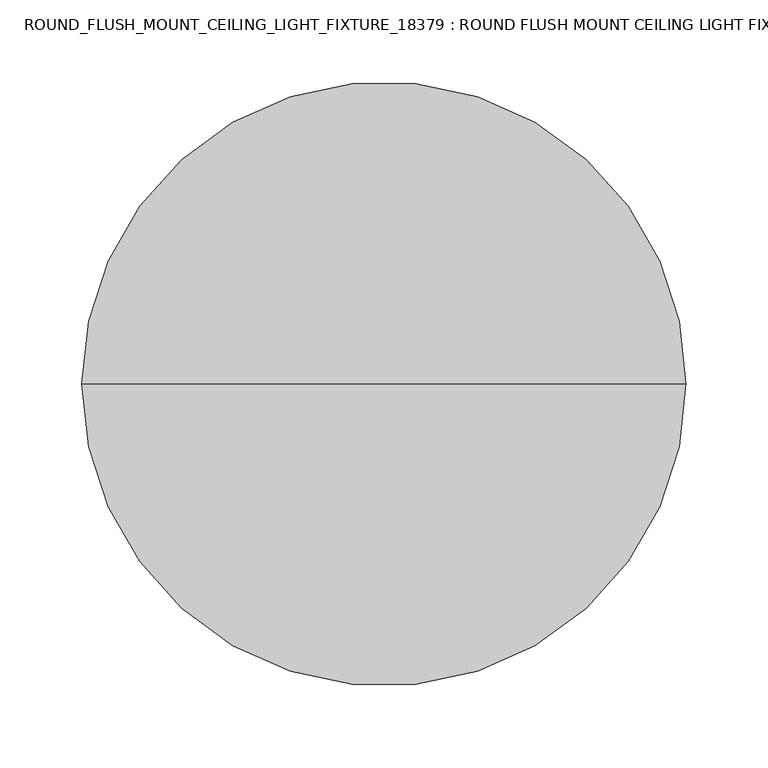
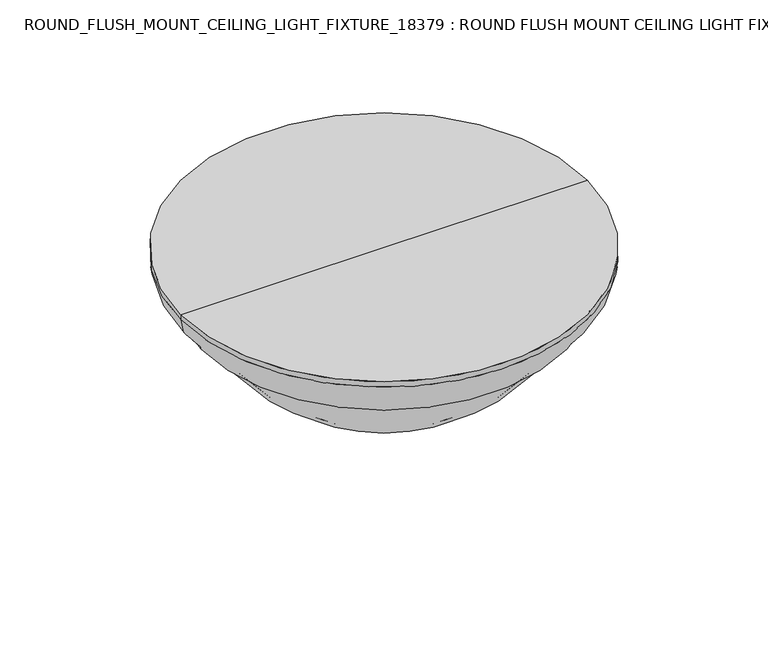
"""IFC4 building model written with IfcOpenShell, lengths in millimetres: light fixture geometry, ROUND_FLUSH_MOUNT_CEILING_LIGHT_FIXTURE_18379 : ROUND FLUSH MOUNT CEILING LIGHT FIXTURE."""

from ifc_helpers import new_model, si_unit, point, frame, origin, place, context, project, spatial, polyline, circle_curve, ellipse_curve, trimmed, source, transform, mapped, element, save
from ifc_brep_helpers import plane_surface, cylinder_surface, revolved_surface, spline_curve, advanced_brep


def round_flush_mount_ceiling_light_fixture_18379_round_flush_30de1430(model_context):
    return source(origin(), model_context, "Body", "AdvancedBrep", [
        advanced_brep(
        [(0.0, 0.0, 2438.4), (184.15, 0.0, 2438.4), (-184.15, 0.0, 2438.4), (-158.75, 0.0, 2403.475), (158.75, 0.0, 2403.475), (0.0, 0.0, 2403.475), (-158.75, 0.0, 2410.5580198), (158.75, 0.0, 2410.5580198), (-160.6175887, 0.0, 2410.5580198), (160.6175887, 0.0, 2410.5580198), (-160.6175887, 0.0, 2401.4555095), (160.6175887, 0.0, 2401.4555095), (-184.15, 0.0, 2433.2858456), (184.15, 0.0, 2433.2858456)],
        [
            (0, 1),
            (1, 2, circle_curve(frame((0.0, 0.0, 2438.4), z_axis=(0.0, 0.0, 1.0), x_axis=(1.0, 0.0, 0.0)), 184.15)),
            (2, 0),
            (2, 1, circle_curve(frame((0.0, 0.0, 2438.4), z_axis=(0.0, 0.0, 1.0), x_axis=(1.0, 0.0, 0.0)), 184.15)),
            (3, 4, circle_curve(frame((0.0, 0.0, 2403.475), z_axis=(0.0, 0.0, -1.0), x_axis=(1.0, 0.0, 0.0)), 158.75)),
            (4, 5),
            (5, 3),
            (4, 3, circle_curve(frame((0.0, 0.0, 2403.475), z_axis=(0.0, 0.0, -1.0), x_axis=(1.0, 0.0, 0.0)), 158.75)),
            (6, 7, circle_curve(frame((0.0, 0.0, 2410.5580198), z_axis=(0.0, 0.0, -1.0), x_axis=(1.0, 0.0, 0.0)), 158.75)),
            (7, 4),
            (3, 6),
            (7, 6, circle_curve(frame((0.0, 0.0, 2410.5580198), z_axis=(0.0, 0.0, -1.0), x_axis=(1.0, 0.0, 0.0)), 158.75)),
            (8, 9, circle_curve(frame((0.0, 0.0, 2410.5580198), z_axis=(0.0, 0.0, -1.0), x_axis=(1.0, 0.0, 0.0)), 160.6175887)),
            (9, 7),
            (6, 8),
            (9, 8, circle_curve(frame((0.0, 0.0, 2410.5580198), z_axis=(0.0, 0.0, -1.0), x_axis=(1.0, 0.0, 0.0)), 160.6175887)),
            (10, 11, circle_curve(frame((0.0, 0.0, 2401.4555095), z_axis=(0.0, 0.0, -1.0), x_axis=(1.0, 0.0, 0.0)), 160.6175887)),
            (11, 9),
            (8, 10),
            (11, 10, circle_curve(frame((0.0, 0.0, 2401.4555095), z_axis=(0.0, 0.0, -1.0), x_axis=(1.0, 0.0, 0.0)), 160.6175887)),
            (12, 13, circle_curve(frame((0.0, 0.0, 2433.2858456), z_axis=(0.0, 0.0, -1.0), x_axis=(1.0, 0.0, 0.0)), 184.15)),
            (13, 11, spline_curve(3, [(184.15, 0.0, 2433.2858456), (183.615320385, 0.0, 2427.010384292), (182.802222876, 0.0, 2424.091263675), (181.092522131, 0.0, 2420.009557598), (180.225634333, 0.0, 2418.65220381), (178.375332652, 0.0, 2416.534281347), (177.472642868, 0.0, 2415.708993281), (175.973354403, 0.0, 2415.374038895), (175.350808812, 0.0, 2415.666114844), (174.743721115, 0.0, 2414.934357445), (174.703424758, 0.0, 2414.034750962), (174.373482724, 0.0, 2412.124948651), (174.053723853, 0.0, 2411.114784901), (173.016018236, 0.0, 2409.360954595), (172.322020854, 0.0, 2408.605305587), (170.85800639, 0.0, 2407.80971777), (170.089071715, 0.0, 2407.760774249), (168.822273168, 0.0, 2406.883061657), (168.354122442, 0.0, 2405.986228604), (167.497455726, 0.0, 2403.827219731), (167.105852162, 0.0, 2402.59008844), (166.48489154, 0.0, 2400.825968614), (166.244601797, 0.0, 2400.247707055), (165.705769205, 0.0, 2399.02983051), (165.421452188, 0.0, 2398.41257598), (164.315501634, 0.0, 2397.452273653), (163.489796173, 0.0, 2397.111347979), (162.147725299, 0.0, 2397.205369108), (161.633671356, 0.0, 2397.64602069), (160.852896111, 0.0, 2399.171247687), (160.557413287, 0.0, 2400.112105853), (160.6175887, 0.0, 2401.4555095)], [4, 2, 2, 2, 2, 2, 2, 2, 2, 2, 2, 2, 2, 2, 2, 4], [0.0, 0.019376612157141843, 0.035912684735600664, 0.048393137631931524, 0.05877054632348552, 0.06814685230600583, 0.07867851307443108, 0.08860469270246224, 0.09840428045130534, 0.1090639243334101, 0.11908634730945084, 0.12825988699908072, 0.1360516794948086, 0.14390275883007766, 0.15181137950200543, 0.15816429510734129])),
            (10, 12, spline_curve(3, [(-160.6175887, 0.0, 2401.4555095), (-160.557413287, 0.0, 2400.112105853), (-160.852896111, 0.0, 2399.171247687), (-161.633671356, 0.0, 2397.64602069), (-162.147725299, 0.0, 2397.205369108), (-163.489796173, 0.0, 2397.111347979), (-164.315501634, 0.0, 2397.452273653), (-165.421452188, 0.0, 2398.41257598), (-165.705769205, 0.0, 2399.02983051), (-166.244601797, 0.0, 2400.247707055), (-166.48489154, 0.0, 2400.825968614), (-167.105852162, 0.0, 2402.59008844), (-167.497455726, 0.0, 2403.827219731), (-168.354122442, 0.0, 2405.986228604), (-168.822273168, 0.0, 2406.883061657), (-170.089071715, 0.0, 2407.760774249), (-170.85800639, 0.0, 2407.80971777), (-172.322020854, 0.0, 2408.605305587), (-173.016018236, 0.0, 2409.360954595), (-174.053723853, 0.0, 2411.114784901), (-174.373482724, 0.0, 2412.124948651), (-174.703424758, 0.0, 2414.034750962), (-174.743721115, 0.0, 2414.934357445), (-175.350808812, 0.0, 2415.666114844), (-175.973354403, 0.0, 2415.374038895), (-177.472642868, 0.0, 2415.708993281), (-178.375332652, 0.0, 2416.534281347), (-180.225634333, 0.0, 2418.65220381), (-181.092522131, 0.0, 2420.009557598), (-182.802222876, 0.0, 2424.091263675), (-183.615320385, 0.0, 2427.010384292), (-184.15, 0.0, 2433.2858456)], [4, 2, 2, 2, 2, 2, 2, 2, 2, 2, 2, 2, 2, 2, 2, 4], [0.0, 0.0063529156053358515, 0.01426153627726362, 0.022112615612532693, 0.02990440810826056, 0.03907794779789045, 0.04910037077393119, 0.05976001465603595, 0.06955960240487905, 0.07948578203291021, 0.09001744280133546, 0.09939374878385576, 0.10977115747540976, 0.12225161037174062, 0.13878768295019944, 0.15816429510734129])),
            (13, 12, circle_curve(frame((0.0, 0.0, 2433.2858456), z_axis=(0.0, 0.0, -1.0), x_axis=(1.0, 0.0, 0.0)), 184.15)),
            (1, 13),
            (12, 2),
        ],
        [
            plane_surface(frame((0.0, 0.0, 2438.4), z_axis=(0.0, 0.0, 1.0), x_axis=(1.0, 0.0, 0.0))),
            plane_surface(frame((0.0, 0.0, 2403.475), z_axis=(0.0, 0.0, -1.0), x_axis=(1.0, 0.0, 0.0))),
            cylinder_surface(frame((0.0, 0.0, 2032.0), z_axis=(0.0, 0.0, 1.0), x_axis=(1.0, 0.0, 0.0)), 158.75),
            plane_surface(frame((0.0, 0.0, 2410.5580198), z_axis=(0.0, 0.0, -1.0), x_axis=(1.0, 0.0, 0.0))),
            revolved_surface(polyline([(160.6175887, 0.0, 2410.5580198), (160.6175887, 0.0, 2401.4555095)]), (0.0, 0.0, 2032.0), (0.0, 0.0, 1.0)),
            revolved_surface(spline_curve(3, [(160.6175887, 0.0, 2401.4555095), (160.557413287, 0.0, 2400.112105853), (160.852896111, 0.0, 2399.171247687), (161.633671356, 0.0, 2397.64602069), (162.147725299, 0.0, 2397.205369108), (163.489796173, 0.0, 2397.111347979), (164.315501634, 0.0, 2397.452273653), (165.421452188, 0.0, 2398.41257598), (165.705769205, 0.0, 2399.02983051), (166.244601797, 0.0, 2400.247707055), (166.48489154, 0.0, 2400.825968614), (167.105852162, 0.0, 2402.59008844), (167.497455726, 0.0, 2403.827219731), (168.354122442, 0.0, 2405.986228604), (168.822273168, 0.0, 2406.883061657), (170.089071715, 0.0, 2407.760774249), (170.85800639, 0.0, 2407.80971777), (172.322020854, 0.0, 2408.605305587), (173.016018236, 0.0, 2409.360954595), (174.053723853, 0.0, 2411.114784901), (174.373482724, 0.0, 2412.124948651), (174.703424758, 0.0, 2414.034750962), (174.743721115, 0.0, 2414.934357445), (175.350808812, 0.0, 2415.666114844), (175.973354403, 0.0, 2415.374038895), (177.472642868, 0.0, 2415.708993281), (178.375332652, 0.0, 2416.534281347), (180.225634333, 0.0, 2418.65220381), (181.092522131, 0.0, 2420.009557598), (182.802222876, 0.0, 2424.091263675), (183.615320385, 0.0, 2427.010384292), (184.15, 0.0, 2433.2858456)], [4, 2, 2, 2, 2, 2, 2, 2, 2, 2, 2, 2, 2, 2, 2, 4], [0.0, 0.0063529156053358515, 0.01426153627726362, 0.022112615612532693, 0.02990440810826056, 0.03907794779789045, 0.04910037077393119, 0.05976001465603595, 0.06955960240487905, 0.07948578203291021, 0.09001744280133546, 0.09939374878385576, 0.10977115747540976, 0.12225161037174062, 0.13878768295019944, 0.15816429510734129]), (0.0, 0.0, 2032.0), (0.0, 0.0, 1.0)),
            cylinder_surface(frame((0.0, 0.0, 2032.0), z_axis=(0.0, 0.0, 1.0), x_axis=(1.0, 0.0, 0.0)), 184.15),
        ],
        [
            (0, [[1, 2, 3]]),
            (0, [[-3, 4, -1]]),
            (1, [[5, 6, 7]]),
            (1, [[8, -7, -6]]),
            (2, [[9, 10, -5, 11]]),
            (2, [[12, -11, -8, -10]]),
            (3, [[13, 14, -9, 15]]),
            (3, [[16, -15, -12, -14]]),
            (4, [[17, 18, -13, 19]]),
            (4, [[20, -19, -16, -18]]),
            (5, [[21, 22, -17, 23]]),
            (5, [[24, -23, -20, -22]]),
            (6, [[-2, 25, -21, 26]]),
            (6, [[-4, -26, -24, -25]]),
        ],
    ),
        advanced_brep(
        [(-158.75, 0.0, 2410.5580198), (158.75, 0.0, 2410.5580198), (158.75, 0.0, 2402.1307288), (-158.75, 0.0, 2402.1307288), (-156.4070964, 0.0, 2410.5580198), (156.4070964, 0.0, 2410.5580198), (-156.4070964, 0.0, 2403.2112109), (156.4070964, 0.0, 2403.2112109), (0.0, 0.0, 2301.2412867), (0.0, 0.0, 2298.6615992)],
        [
            (0, 1, circle_curve(frame((0.0, 0.0, 2410.5580198), z_axis=(0.0, 0.0, -1.0), x_axis=(1.0, 0.0, 0.0)), 158.75)),
            (1, 2),
            (2, 3, circle_curve(frame((0.0, 0.0, 2402.1307288), z_axis=(0.0, 0.0, 1.0), x_axis=(1.0, 0.0, 0.0)), 158.75)),
            (3, 0),
            (1, 0, circle_curve(frame((0.0, 0.0, 2410.5580198), z_axis=(0.0, 0.0, -1.0), x_axis=(1.0, 0.0, 0.0)), 158.75)),
            (3, 2, circle_curve(frame((0.0, 0.0, 2402.1307288), z_axis=(0.0, 0.0, 1.0), x_axis=(1.0, 0.0, 0.0)), 158.75)),
            (4, 5, circle_curve(frame((0.0, 0.0, 2410.5580198), z_axis=(0.0, 0.0, -1.0), x_axis=(1.0, 0.0, 0.0)), 156.4070964)),
            (5, 1),
            (0, 4),
            (5, 4, circle_curve(frame((0.0, 0.0, 2410.5580198), z_axis=(0.0, 0.0, -1.0), x_axis=(1.0, 0.0, 0.0)), 156.4070964)),
            (6, 7, circle_curve(frame((0.0, 0.0, 2403.2112109), z_axis=(0.0, 0.0, -1.0), x_axis=(1.0, 0.0, 0.0)), 156.4070964)),
            (7, 5),
            (4, 6),
            (7, 6, circle_curve(frame((0.0, 0.0, 2403.2112109), z_axis=(0.0, 0.0, -1.0), x_axis=(1.0, 0.0, 0.0)), 156.4070964)),
            (8, 7, circle_curve(frame((0.0, 0.0, 2472.1791663), z_axis=(0.0, -1.0, 0.0), x_axis=(0.0, 0.0, -1.0)), 170.9378796)),
            (6, 8, circle_curve(frame((0.0, 0.0, 2472.1791663), z_axis=(0.0, -1.0, 0.0), x_axis=(0.0, 0.0, -1.0)), 170.9378796)),
            (2, 9, circle_curve(frame((0.0, 0.0, 2472.1791663), z_axis=(0.0, 1.0, 0.0), x_axis=(0.0, 0.0, -1.0)), 173.5175671)),
            (9, 3, circle_curve(frame((0.0, 0.0, 2472.1791663), z_axis=(0.0, 1.0, 0.0), x_axis=(0.0, 0.0, -1.0)), 173.5175671)),
        ],
        [
            cylinder_surface(frame((0.0, 0.0, 2032.0), z_axis=(0.0, 0.0, 1.0), x_axis=(1.0, 0.0, 0.0)), 158.75),
            plane_surface(frame((0.0, 0.0, 2410.5580198), z_axis=(0.0, 0.0, 1.0), x_axis=(1.0, 0.0, 0.0))),
            revolved_surface(polyline([(156.4070964, 0.0, 2410.5580198), (156.4070964, 0.0, 2403.2112109)]), (0.0, 0.0, 2032.0), (0.0, 0.0, 1.0)),
            revolved_surface(trimmed(ellipse_curve(frame((0.0, 0.0, 2472.1791663), z_axis=(0.0, 1.0, 0.0), x_axis=(0.0, 0.0, -1.0)), 170.9378796, 170.9378796), [point((156.4070964, 0.0, 2403.2112109))], [point((0.0, 0.0, 2301.2412867))], True, "CARTESIAN"), (0.0, 0.0, 2032.0), (0.0, 0.0, 1.0)),
            revolved_surface(trimmed(ellipse_curve(frame((0.0, 0.0, 2472.1791663), z_axis=(0.0, -1.0, 0.0), x_axis=(0.0, 0.0, -1.0)), 173.5175671, 173.5175671), [point((0.0, 0.0, 2298.6615992))], [point((158.75, 0.0, 2402.1307288))], True, "CARTESIAN"), (0.0, 0.0, 2032.0), (0.0, 0.0, 1.0)),
        ],
        [
            (0, [[1, 2, 3, 4]]),
            (0, [[5, -4, 6, -2]]),
            (1, [[7, 8, -1, 9]]),
            (1, [[10, -9, -5, -8]]),
            (2, [[11, 12, -7, 13]]),
            (2, [[14, -13, -10, -12]]),
            (3, [[15, -11, 16]]),
            (3, [[-16, -14, -15]]),
            (4, [[-3, 17, 18]]),
            (4, [[-6, -18, -17]]),
        ],
    ),
        advanced_brep(
        [(0.0, 0.0, 2299.0088232), (18.8438581, 0.0, 2300.0350713), (-18.8438581, 0.0, 2300.0350713), (-18.8438581, 0.0, 2296.3917407), (18.8438581, 0.0, 2296.3917407), (0.0, 0.0, 2273.6088232)],
        [
            (0, 1, circle_curve(frame((0.0, 0.0, 2472.5263903), z_axis=(0.0, -1.0, 0.0), x_axis=(0.0, 0.0, -1.0)), 173.5175671)),
            (1, 2, circle_curve(frame((0.0, 0.0, 2300.0350713), z_axis=(0.0, 0.0, 1.0), x_axis=(1.0, 0.0, 0.0)), 18.8438581)),
            (2, 0, circle_curve(frame((0.0, 0.0, 2472.5263903), z_axis=(0.0, -1.0, 0.0), x_axis=(0.0, 0.0, -1.0)), 173.5175671)),
            (2, 1, circle_curve(frame((0.0, 0.0, 2300.0350713), z_axis=(0.0, 0.0, 1.0), x_axis=(1.0, 0.0, 0.0)), 18.8438581)),
            (3, 4, circle_curve(frame((0.0, 0.0, 2296.3917407), z_axis=(0.0, 0.0, -1.0), x_axis=(1.0, 0.0, 0.0)), 18.8438581)),
            (4, 5, spline_curve(3, [(18.8438581, 0.0, 2296.3917407), (18.022484889, 0.0, 2291.682650982), (16.056250154, 0.0, 2289.709138675), (12.58639441, 0.0, 2287.577694333), (11.060444469, 0.0, 2287.305720814), (8.404841494, 0.0, 2286.44406903), (7.249521242, 0.0, 2285.902733904), (5.949325353, 0.0, 2284.0821281), (5.652366033, 0.0, 2282.965615023), (5.850726514, 0.0, 2281.317666152), (6.200668977, 0.0, 2280.714125509), (7.046725778, 0.0, 2279.826890077), (7.542284271, 0.0, 2279.541998515), (7.902687498, 0.0, 2278.290807244), (7.535084472, 0.0, 2277.146478307), (5.264094118, 0.0, 2274.80244107), (3.168441017, 0.0, 2273.614676074), (0.0, 0.0, 2273.6088232)], [4, 2, 2, 2, 2, 2, 2, 2, 4], [0.0, 0.016116581655971948, 0.031140280999285994, 0.044116736851914314, 0.054586381593721686, 0.0629807388696783, 0.07134346095475164, 0.08220267457229385, 0.09446473776260068])),
            (5, 3, spline_curve(3, [(0.0, 0.0, 2273.6088232), (-3.168441017, 0.0, 2273.614676074), (-5.264094118, 0.0, 2274.80244107), (-7.535084472, 0.0, 2277.146478307), (-7.902687498, 0.0, 2278.290807244), (-7.542284271, 0.0, 2279.541998515), (-7.046725778, 0.0, 2279.826890077), (-6.200668977, 0.0, 2280.714125509), (-5.850726514, 0.0, 2281.317666152), (-5.652366033, 0.0, 2282.965615023), (-5.949325353, 0.0, 2284.0821281), (-7.249521242, 0.0, 2285.902733904), (-8.404841494, 0.0, 2286.44406903), (-11.060444469, 0.0, 2287.305720814), (-12.58639441, 0.0, 2287.577694333), (-16.056250154, 0.0, 2289.709138675), (-18.022484889, 0.0, 2291.682650982), (-18.8438581, 0.0, 2296.3917407)], [4, 2, 2, 2, 2, 2, 2, 2, 4], [0.0, 0.01226206319030683, 0.023121276807849048, 0.03148399889292239, 0.039878356168879, 0.05034800091068637, 0.06332445676331469, 0.07834815610662874, 0.09446473776260068])),
            (4, 3, circle_curve(frame((0.0, 0.0, 2296.3917407), z_axis=(0.0, 0.0, -1.0), x_axis=(1.0, 0.0, 0.0)), 18.8438581)),
            (1, 4),
            (3, 2),
        ],
        [
            revolved_surface(trimmed(ellipse_curve(frame((0.0, 0.0, 2472.5263903), z_axis=(0.0, 1.0, 0.0), x_axis=(0.0, 0.0, -1.0)), 173.5175671, 173.5175671), [point((18.8438581, 0.0, 2300.0350713))], [point((0.0, 0.0, 2299.0088232))], True, "CARTESIAN"), (0.0, 0.0, 2032.0), (0.0, 0.0, 1.0)),
            revolved_surface(spline_curve(3, [(0.0, 0.0, 2273.6088232), (3.168441017, 0.0, 2273.614676074), (5.264094118, 0.0, 2274.80244107), (7.535084472, 0.0, 2277.146478307), (7.902687498, 0.0, 2278.290807244), (7.542284271, 0.0, 2279.541998515), (7.046725778, 0.0, 2279.826890077), (6.200668977, 0.0, 2280.714125509), (5.850726514, 0.0, 2281.317666152), (5.652366033, 0.0, 2282.965615023), (5.949325353, 0.0, 2284.0821281), (7.249521242, 0.0, 2285.902733904), (8.404841494, 0.0, 2286.44406903), (11.060444469, 0.0, 2287.305720814), (12.58639441, 0.0, 2287.577694333), (16.056250154, 0.0, 2289.709138675), (18.022484889, 0.0, 2291.682650982), (18.8438581, 0.0, 2296.3917407)], [4, 2, 2, 2, 2, 2, 2, 2, 4], [0.0, 0.01226206319030683, 0.023121276807849048, 0.03148399889292239, 0.039878356168879, 0.05034800091068637, 0.06332445676331469, 0.07834815610662874, 0.09446473776260068]), (0.0, 0.0, 2032.0), (0.0, 0.0, 1.0)),
            cylinder_surface(frame((0.0, 0.0, 2032.0), z_axis=(0.0, 0.0, 1.0), x_axis=(1.0, 0.0, 0.0)), 18.8438581),
        ],
        [
            (0, [[1, 2, 3]]),
            (0, [[-3, 4, -1]]),
            (1, [[5, 6, 7]]),
            (1, [[8, -7, -6]]),
            (2, [[-2, 9, -5, 10]]),
            (2, [[-4, -10, -8, -9]]),
        ],
    ),
    ])


if __name__ == "__main__":
    model = new_model("IFC4")
    model_context = context("Model", 3, world=origin())
    ifc_project = project(units=[si_unit("LENGTHUNIT", "METRE", prefix="MILLI")], contexts=[model_context])
    site = spatial("IfcSite", under=ifc_project)
    building = spatial("IfcBuilding", under=site)
    placement = place(None, origin())
    round_flush_mount_ceiling_light_fixture_18379_round_flush_shape = round_flush_mount_ceiling_light_fixture_18379_round_flush_30de1430(model_context)
    element("IfcLightFixture", 1, ObjectType="ROUND_FLUSH_MOUNT_CEILING_LIGHT_FIXTURE_18379 : ROUND FLUSH MOUNT CEILING LIGHT FIXTURE", at=placement, inside=building, context=model_context, shape_type="MappedRepresentation", body=[
        mapped(round_flush_mount_ceiling_light_fixture_18379_round_flush_shape, transform((0.0, 0.0, 0.0), x_axis=(1.0, 0.0, 0.0), y_axis=(0.0, 1.0, 0.0), z_axis=(0.0, 0.0, 1.0))),
    ])
    save(model, "model.ifc")

# Revit data of these elements
# Type "ROUND_FLUSH_MOUNT_CEILING_LIGHT_FIXTURE_18379 : ROUND FLUSH MOUNT CEILING LIGHT FIXTURE"
#   Wattage = 100 W
#   built-in parameter 1150110 = 1 (stored number, unit not read)
#   built-in parameter 1114217 = 1 (stored number, unit not read)
#   built-in parameter 1150109 = 1 (stored number, unit not read)
#   built-in parameter 1150113 = 1 (stored number, unit not read)
#   STUDIO LIGHT OFFSET [instance default] = 3' - 6"
#   Lumens = 14854.2 lm
#   built-in parameter 1150115 = 1 (stored number, unit not read)
#   built-in parameter 1150105 = 4728.24 (stored number, unit not read)
#   Light Source Symbol Size = 2' - 0"
#   built-in parameter 1150112 = 1 (stored number, unit not read)
#   built-in parameter 1150114 = 1 (stored number, unit not read)
#   built-in parameter 1150107 = 3000 (stored number, unit not read)
#   built-in parameter 1150106 = 47.2824 (stored number, unit not read)
#   built-in parameter 1150104 = 13.8 (stored number, unit not read)
#   built-in parameter 1114218 = 1 (stored number, unit not read)
#   built-in parameter 1150133 = 10 (stored number, unit not read)
#   STUDIO LIGHT [instance default] = yes
#   Color Filter = 16777215
#   Light Fixture Material = Light Fixture
#   Light Fixture Glass = Light Glass
#   Dimming Lamp Color Temperature Shift = (empty or 0)
#   Default Elevation = 0
# Element 1 (IfcLightFixture, "ROUND_FLUSH_MOUNT_CEILING_LIGHT_FIXTURE_18379 : ROUND FLUSH MOUNT CEILING LIGHT FIXTURE")
#   Materials on its faces: "Light Fixture", "Light Glass"
# Materials
#   "Light Fixture": class "Generic", colour RGB 105 77 58, transparency 0, Cost = 0
#   "Light Glass": class "Generic", colour RGB 242 242 242, transparency 1, Cost = 0
